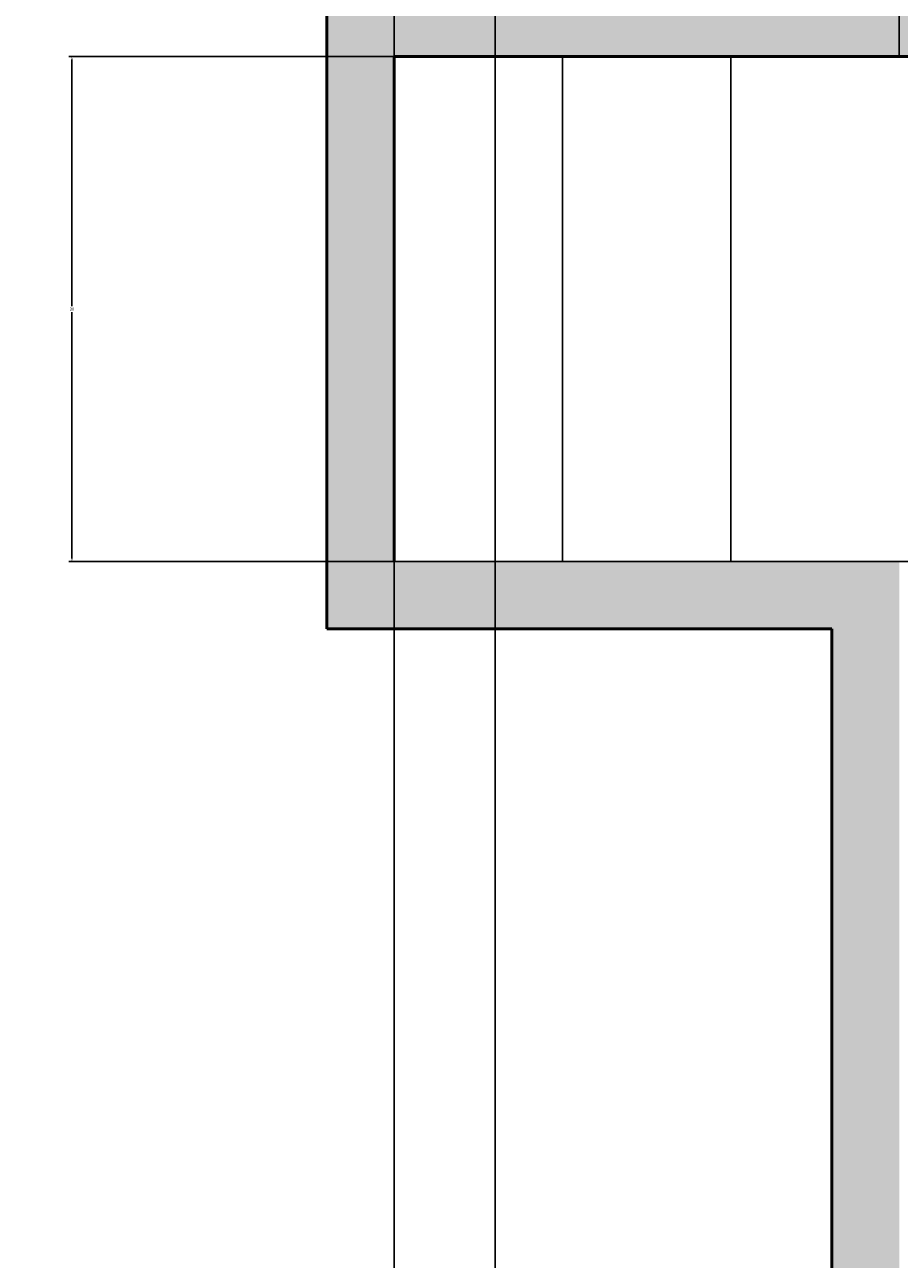
# Model space of a CAD drawing. Units: inches. Extents: x 2307 to 2544, y 2171 to 2540.
# Tile 13 of 52: x 2434 to 2486, y 2244 to 2317. Entities that reach past the tile are written whole.
import ezdxf

# ---------------------------------------------------------------- set-up
doc = ezdxf.new("R2010")
doc.units = ezdxf.units.IN
for name, color, linetype, lineweight in [('A-ANNO-DIMS', 2, 'Continuous', 18), ('A-FLOR-STRS', 7, 'Continuous', 25), ('A-WALL', 7, 'Continuous', 50)]:
    doc.layers.add(name, color=color, linetype=linetype, lineweight=lineweight)
doc.layers.add('A-WALL-PATT', color=18, linetype='Continuous', lineweight=13, true_color=0x000000)
doc.styles.get("Standard").update_dxf_attribs({"font": 'arial.ttf'})
doc.dimstyles.get("Standard").update_dxf_attribs({"dimtxt": 0.18, "dimasz": 0.18, "dimexe": 0.18, "dimexo": 0.0625, "dimgap": 0.09, "dimtad": 0, "dimtih": 1, "dimtoh": 1, "dimdec": 4, "dimzin": 0, "dimdsep": 46, "dimtxsty": 'Standard', "dimcen": 0.09, "dimadec": 0, "dimazin": 0, "dimtfac": 1, "dimtdec": 4, "dimtofl": 0, "dimtmove": 0, "dimatfit": 3, "dimfxl": 1, "dimtolj": 1, "dimtzin": 0, "dimarcsym": 0})

# ---------------------------------------------------------------- blocks, each defined once
blk = doc.blocks.new('*D53')
at = {"layer": 'A-ANNO-DIMS', "color": 0, "lineweight": -2, "transparency": 16777216}
for p, q in [((2455.696, 2439.447), (2455.696, 2171.18)), ((2461.696, 2439.447), (2461.696, 2171.18)), ((2455.876, 2171.36), (2458.546, 2171.36)), ((2461.516, 2171.36), (2458.845, 2171.36))]:
    blk.add_line(p, q, dxfattribs=at)
at = {"layer": 'A-ANNO-DIMS', "color": 0, "transparency": 16777216}
for points in [[(2455.876, 2171.39), (2455.876, 2171.33), (2455.696, 2171.36)], [(2461.516, 2171.39), (2461.516, 2171.33), (2461.696, 2171.36)]]:
    blk.add_solid(points, dxfattribs=at)
at = {"layer": 'Defpoints', "color": 0, "transparency": 16777216}
for p in [(2455.696, 2439.51), (2461.696, 2439.51), (2461.696, 2171.36)]:
    blk.add_point(p, dxfattribs=at)
at = {"layer": 'A-ANNO-DIMS', "color": 0, "transparency": 16777216, "insert": (2458.696, 2171.36), "char_height": 0.18, "attachment_point": 5}
blk.add_mtext('\\A1;6', dxfattribs=at)
blk = doc.blocks.new('*D54')
at = {"layer": 'A-ANNO-DIMS', "color": 0, "lineweight": -2, "transparency": 16777216}
for p, q in [((2461.696, 2435.447), (2461.696, 2171.18)), ((2491.696, 2435.447), (2491.696, 2171.18)), ((2461.876, 2171.36), (2476.477, 2171.36)), ((2491.516, 2171.36), (2476.914, 2171.36))]:
    blk.add_line(p, q, dxfattribs=at)
at = {"layer": 'A-ANNO-DIMS', "color": 0, "transparency": 16777216}
for points in [[(2461.876, 2171.39), (2461.876, 2171.33), (2461.696, 2171.36)], [(2491.516, 2171.39), (2491.516, 2171.33), (2491.696, 2171.36)]]:
    blk.add_solid(points, dxfattribs=at)
at = {"layer": 'Defpoints', "color": 0, "transparency": 16777216}
for p in [(2461.696, 2435.51), (2491.696, 2435.51), (2491.696, 2171.36)]:
    blk.add_point(p, dxfattribs=at)
at = {"layer": 'A-ANNO-DIMS', "color": 0, "transparency": 16777216, "insert": (2476.696, 2171.36), "char_height": 0.18, "attachment_point": 5}
blk.add_mtext('\\A1;30', dxfattribs=at)
blk = doc.blocks.new('*D57')
at = {"layer": 'A-ANNO-DIMS', "color": 0, "lineweight": -2, "transparency": 16777216}
for p, q in [((2455.633, 2315.51), (2436.366, 2315.51)), ((2436.546, 2315.33), (2436.546, 2300.692)), ((2436.546, 2285.69), (2436.546, 2300.328)), ((2455.633, 2285.51), (2436.366, 2285.51))]:
    blk.add_line(p, q, dxfattribs=at)
at = {"layer": 'A-ANNO-DIMS', "color": 0, "transparency": 16777216}
for points in [[(2436.516, 2315.33), (2436.576, 2315.33), (2436.546, 2315.51)], [(2436.516, 2285.69), (2436.576, 2285.69), (2436.546, 2285.51)]]:
    blk.add_solid(points, dxfattribs=at)
at = {"layer": 'Defpoints', "color": 0, "transparency": 16777216}
for p in [(2436.546, 2315.51), (2455.696, 2315.51), (2455.696, 2285.51)]:
    blk.add_point(p, dxfattribs=at)
at = {"layer": 'A-ANNO-DIMS', "color": 0, "transparency": 16777216, "insert": (2436.546, 2300.51), "char_height": 0.18, "attachment_point": 5}
blk.add_mtext('\\A1;30', dxfattribs=at)
blk = doc.blocks.new('*D59')
at = {"layer": 'A-ANNO-DIMS', "color": 0, "lineweight": -2, "transparency": 16777216}
for p, q in [((2455.696, 2315.572), (2455.696, 2540.345)), ((2455.876, 2540.165), (2470.477, 2540.165)), ((2485.516, 2540.165), (2470.914, 2540.165)), ((2485.696, 2315.572), (2485.696, 2540.345))]:
    blk.add_line(p, q, dxfattribs=at)
at = {"layer": 'A-ANNO-DIMS', "color": 0, "transparency": 16777216}
for points in [[(2455.876, 2540.195), (2455.876, 2540.135), (2455.696, 2540.165)], [(2485.516, 2540.195), (2485.516, 2540.135), (2485.696, 2540.165)]]:
    blk.add_solid(points, dxfattribs=at)
at = {"layer": 'Defpoints', "color": 0, "transparency": 16777216}
for p in [(2455.696, 2540.165), (2455.696, 2315.51), (2485.696, 2315.51)]:
    blk.add_point(p, dxfattribs=at)
at = {"layer": 'A-ANNO-DIMS', "color": 0, "transparency": 16777216, "insert": (2470.696, 2540.165), "char_height": 0.18, "attachment_point": 5}
blk.add_mtext('\\A1;30', dxfattribs=at)

msp = doc.modelspace()

# ---------------------------------------------------------------- hatches: boundary and pattern name
at = {"layer": 'A-WALL-PATT'}
h = msp.add_hatch(color=256, dxfattribs=at)
h.dxf.hatch_style = 1
h.paths.add_polyline_path([(2433.6935, 2199.5096), (2415.6423, 2199.5096), (2415.6423, 2190.5096), (2433.7832, 2190.5096)], flags=17)
h.paths.add_polyline_path([(2367.6423, 2199.5096), (2335.6958, 2199.5096), (2335.6958, 2307.3983), (2326.6958, 2307.3983), (2326.6958, 2190.5096), (2367.6423, 2190.5096)])
h.paths.add_polyline_path([(2524.6958, 2520.5096), (2496.7832, 2520.5096), (2496.7832, 2515.5149), (2472.7832, 2515.5149), (2472.7832, 2520.5096), (2415.4028, 2520.5096), (2415.4028, 2511.5096), (2451.6958, 2511.5096), (2451.6958, 2439.5096), (2451.6958, 2391.5096), (2445.6958, 2391.5096), (2445.6958, 2387.5096), (2455.6958, 2387.5096), (2455.6958, 2435.5096), (2461.6958, 2435.5096), (2461.6958, 2439.5096), (2455.6958, 2439.5096), (2455.6958, 2511.5096), (2515.6958, 2511.5096), (2515.6958, 2439.5096), (2491.6958, 2439.5096), (2491.6958, 2435.5096), (2515.6958, 2435.5096), (2515.6958, 2319.5096), (2451.6958, 2319.5096), (2451.6958, 2281.5096), (2481.6958, 2281.5096), (2481.6958, 2225.5096), (2485.6958, 2225.5096), (2485.6958, 2285.5096), (2455.6958, 2285.5096), (2455.6958, 2315.5096), (2515.6958, 2315.5096), (2515.6958, 2199.5096), (2469.6952, 2199.5096), (2469.785, 2190.5096), (2524.6958, 2190.5096)])

# ---------------------------------------------------------------- linework, layer by layer
at = {"layer": 'A-FLOR-STRS'}
for p, q in [((2465.6958, 2315.5096), (2465.6958, 2285.5096)), ((2475.6958, 2315.5096), (2475.6958, 2285.5096)), ((2515.6958, 2285.5096), (2455.6958, 2285.5096))]:
    msp.add_line(p, q, dxfattribs=at)
at = {"layer": 'A-WALL'}
for p, q in [((2451.6958, 2319.5096), (2451.6958, 2281.5096)), ((2515.6958, 2315.5096), (2455.6958, 2315.5096)), ((2455.6958, 2315.5096), (2455.6958, 2285.5096)), ((2481.6958, 2281.5096), (2451.6958, 2281.5096)), ((2481.6958, 2281.5096), (2481.6958, 2225.5096))]:
    msp.add_line(p, q, dxfattribs=at)

# ---------------------------------------------------------------- dimensions: what is measured, and where the dimension line sits
at = {"layer": 'A-ANNO-DIMS'}
for base, p1, p2, picture, middle in [((2455.6958, 2540.1649), (2485.6958, 2315.5096), (2455.6958, 2315.5096), '*D59', (2470.6958, 2540.1649)), ((2461.6958, 2171.3596), (2455.6958, 2439.5096), (2461.6958, 2439.5096), '*D53', (2458.6958, 2171.3596)), ((2491.6958, 2171.3596), (2461.6958, 2435.5096), (2491.6958, 2435.5096), '*D54', (2476.6958, 2171.3596))]:
    dim = msp.add_linear_dim(base=base, p1=p1, p2=p2, dimstyle='Standard', override={"dimdec": 0, "dimlfac": 1, "dimrnd": 0, "dimzin": 0, "dimdsep": 46, "dimlunit": 2}, dxfattribs=at)
    dim.commit()
    dim.dimension.update_dxf_attribs({"geometry": picture, "text_midpoint": middle})
dim = msp.add_linear_dim(base=(2436.5458, 2315.5096), p1=(2455.6958, 2285.5096), p2=(2455.6958, 2315.5096), angle=90, dimstyle='Standard', override={"dimdec": 0, "dimlfac": 1, "dimrnd": 0, "dimzin": 0, "dimdsep": 46, "dimlunit": 2}, dxfattribs=at)
dim.commit()
dim.dimension.update_dxf_attribs({"geometry": '*D57', "text_midpoint": (2436.5458, 2300.5096)})

doc.saveas('drawing.dxf')
